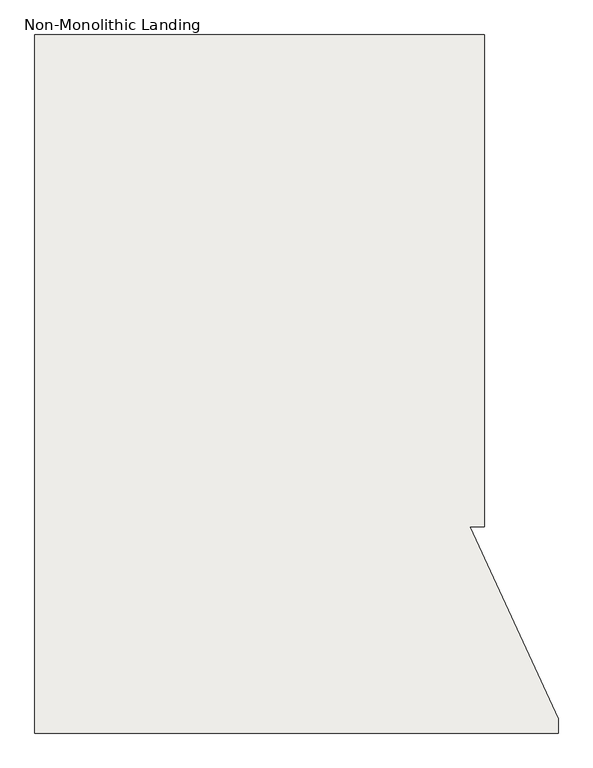
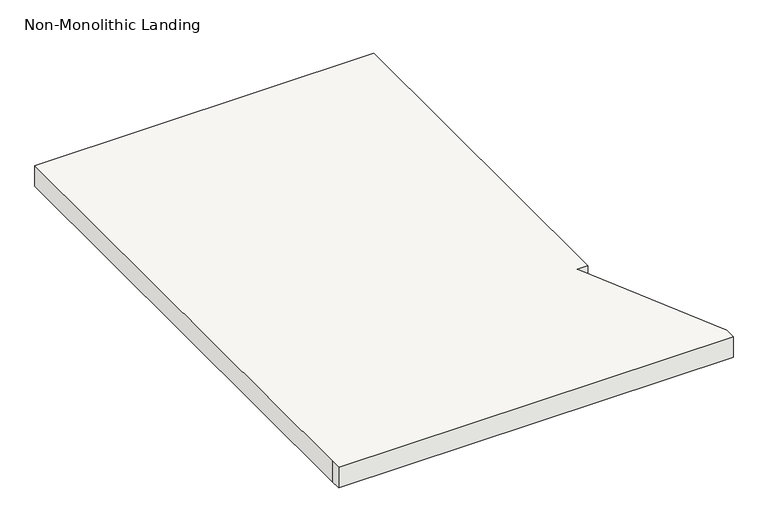
"""IFC4 building model written with IfcOpenShell, lengths in millimetres: slab geometry, Non-Monolithic Landing."""

from ifc_helpers import new_model, si_unit, origin, place, context, project, spatial, faceted_brep, source, transform, mapped, element, save


def non_monolithic_landing_fae4903c(model_context):
    return source(origin(), model_context, "Body", "Brep", [
        faceted_brep([(-9813.5920073, 3951.9968929, 1504.95), (-9813.5920073, 3951.9968929, 1524.0), (-9838.9920073, 3951.9968929, 1524.0), (-9838.9920073, 3951.9968929, 1479.55), (-9813.5920073, 4811.1398463, 1504.95), (-9813.5920073, 4811.1398463, 1524.0), (-9838.9920073, 4811.1398463, 1479.55), (-10599.5602428, 4811.1398463, 1524.0), (-10599.5602428, 3617.3398463, 1524.0), (-10599.5602428, 3591.9398463, 1524.0), (-9685.1602428, 3591.9398463, 1524.0), (-9685.1602428, 3617.3398463, 1524.0), (-9838.9920073, 4811.1398463, 1473.2), (-9838.9920073, 3951.9968929, 1473.2), (-9685.1602428, 3617.3398463, 1473.2), (-9685.1602428, 3591.9398463, 1473.2), (-10599.5602428, 3591.9398463, 1473.2), (-10599.5602428, 3617.3398463, 1473.2), (-10599.5602428, 4811.1398463, 1473.2)], [[[0, 1, 2, 3]], [[4, 5, 1, 0]], [[6, 4, 0, 3]], [[7, 8, 9, 10, 11, 2, 1, 5]], [[12, 13, 14, 15, 16, 17, 18]], [[13, 12, 6, 3]], [[7, 5, 4, 6, 12, 18]], [[8, 7, 18, 17]], [[9, 8, 17, 16]], [[10, 9, 16, 15]], [[11, 10, 15, 14]], [[2, 11, 14, 13, 3]]]),
    ])


if __name__ == "__main__":
    model = new_model("IFC4")
    model_context = context("Model", 3, world=origin())
    ifc_project = project(units=[si_unit("LENGTHUNIT", "METRE", prefix="MILLI")], contexts=[model_context])
    site = spatial("IfcSite", under=ifc_project)
    building = spatial("IfcBuilding", under=site)
    placement = place(None, origin())
    non_monolithic_landing_shape = non_monolithic_landing_fae4903c(model_context)
    element("IfcSlab", 1, ObjectType="Non-Monolithic Landing", at=placement, inside=building, context=model_context, shape_type="MappedRepresentation", body=[
        mapped(non_monolithic_landing_shape, transform((0.0, 0.0, 0.0), x_axis=(1.0, 0.0, 0.0), y_axis=(0.0, 1.0, 0.0), z_axis=(0.0, 0.0, 1.0))),
    ])
    save(model, "model.ifc")
